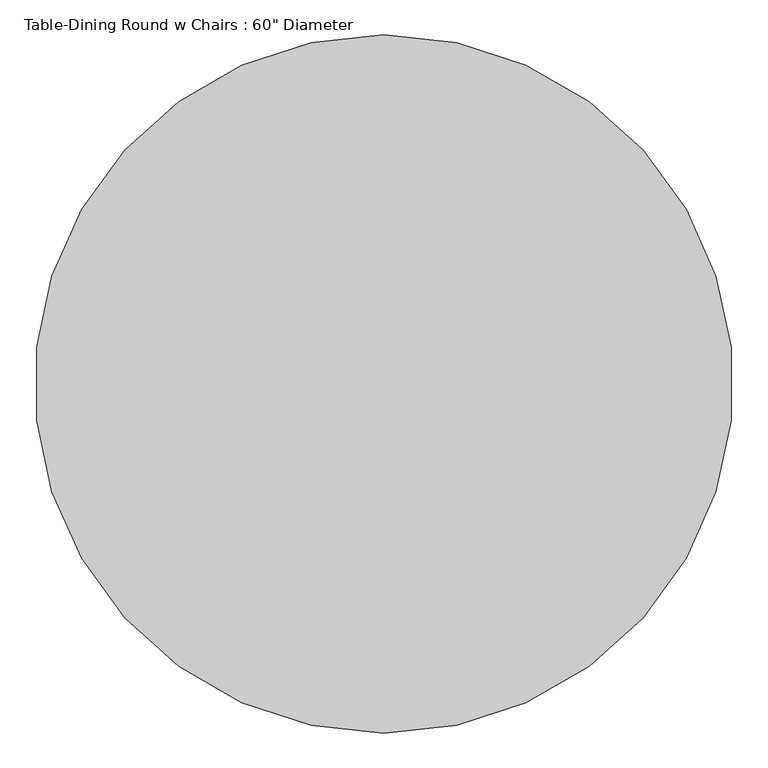
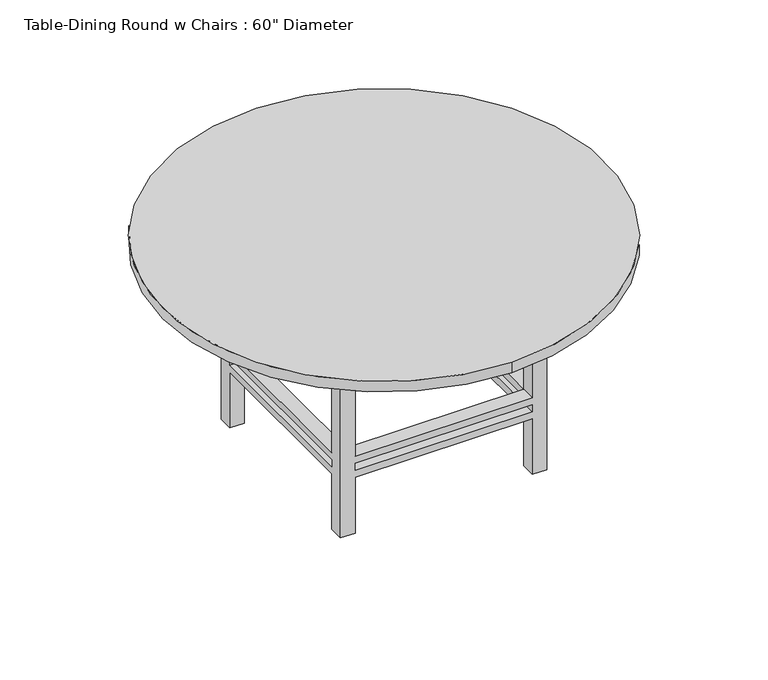
"""IFC4 building model written with IfcOpenShell, lengths in millimetres: furniture geometry."""

from ifc_helpers import new_model, si_unit, point, frame, frame_2d, origin, place, context, project, spatial, polyline, circle_curve, trimmed, segment, composite_curve, outline, extrude, faceted_brep, source, transform, mapped, element, save


def furniture_86cdcdde(model_context):
    return source(origin(), model_context, "Body", "SolidModel", [
        extrude(outline(polyline([(484.6819672, 196.1213115), (484.6819672, -565.8786885), (-277.3180328, -565.8786885), (-277.3180328, 196.1213115), (484.6819672, 196.1213115)]), holes=[polyline([(459.2819672, 170.7213115), (-251.9180328, 170.7213115), (-251.9180328, -540.4786885), (459.2819672, -540.4786885), (459.2819672, 170.7213115)])]), frame((0.0, 0.0, 647.7), z_axis=(0.0, 0.0, 1.0), x_axis=(1.0, 0.0, 0.0)), (0.0, 0.0, 1.0), 76.2),
        faceted_brep([(408.4819672, 119.9213115, 279.4), (408.4819672, -489.6786885, 279.4), (459.2819672, -489.6786885, 279.4), (459.2819672, 119.9213115, 279.4), (-201.1180328, -489.6786885, 279.4), (-201.1180328, -540.4786885, 279.4), (408.4819672, -540.4786885, 279.4), (-201.1180328, 119.9213115, 279.4), (-251.9180328, 119.9213115, 279.4), (-251.9180328, -489.6786885, 279.4), (408.4819672, 170.7213115, 279.4), (-201.1180328, 170.7213115, 279.4), (408.4819672, 119.9213115, 254.0), (-201.1180328, 119.9213115, 254.0), (-201.1180328, 170.7213115, 254.0), (408.4819672, 170.7213115, 254.0), (-201.1180328, -489.6786885, 254.0), (-251.9180328, -489.6786885, 254.0), (-251.9180328, 119.9213115, 254.0), (408.4819672, -489.6786885, 254.0), (408.4819672, -540.4786885, 254.0), (-201.1180328, -540.4786885, 254.0), (459.2819672, 119.9213115, 254.0), (459.2819672, -489.6786885, 254.0), (-251.9180328, 170.7213115, 647.7), (-201.1180328, 170.7213115, 647.7), (408.4819672, 170.7213115, 647.7), (459.2819672, 170.7213115, 647.7), (459.2819672, 170.7213115, 0.0), (408.4819672, 170.7213115, 0.0), (408.4819672, 170.7213115, 203.2), (-201.1180328, 170.7213115, 203.2), (-201.1180328, 170.7213115, 0.0), (-251.9180328, 170.7213115, 0.0), (-201.1180328, 170.7213115, 228.6), (408.4819672, 170.7213115, 228.6), (-251.9180328, 119.9213115, 647.7), (-251.9180328, 119.9213115, 0.0), (-251.9180328, 119.9213115, 203.2), (-251.9180328, -489.6786885, 203.2), (-251.9180328, -489.6786885, 0.0), (-251.9180328, -540.4786885, 0.0), (-251.9180328, -540.4786885, 647.7), (-251.9180328, -489.6786885, 647.7), (-251.9180328, -489.6786885, 228.6), (-251.9180328, 119.9213115, 228.6), (459.2819672, -540.4786885, 647.7), (408.4819672, -540.4786885, 647.7), (-201.1180328, -540.4786885, 647.7), (-201.1180328, -540.4786885, 0.0), (-201.1180328, -540.4786885, 203.2), (408.4819672, -540.4786885, 203.2), (408.4819672, -540.4786885, 0.0), (459.2819672, -540.4786885, 0.0), (408.4819672, -540.4786885, 228.6), (-201.1180328, -540.4786885, 228.6), (459.2819672, 119.9213115, 647.7), (459.2819672, -489.6786885, 647.7), (459.2819672, -489.6786885, 0.0), (459.2819672, -489.6786885, 203.2), (459.2819672, 119.9213115, 203.2), (459.2819672, 119.9213115, 0.0), (459.2819672, 119.9213115, 228.6), (459.2819672, -489.6786885, 228.6), (-201.1180328, 119.9213115, 647.7), (408.4819672, -489.6786885, 647.7), (408.4819672, 119.9213115, 647.7), (-201.1180328, -489.6786885, 647.7), (408.4819672, 119.9213115, 0.0), (-201.1180328, -489.6786885, 0.0), (-201.1180328, 119.9213115, 0.0), (408.4819672, -489.6786885, 0.0), (-201.1180328, 119.9213115, 228.6), (-201.1180328, 119.9213115, 203.2), (408.4819672, 119.9213115, 228.6), (408.4819672, 119.9213115, 203.2), (408.4819672, -489.6786885, 228.6), (408.4819672, -489.6786885, 203.2), (-201.1180328, -489.6786885, 228.6), (-201.1180328, -489.6786885, 203.2)], [[[0, 1, 2, 3]], [[1, 4, 5, 6]], [[4, 7, 8, 9]], [[7, 0, 10, 11]], [[12, 13, 14, 15]], [[13, 16, 17, 18]], [[16, 19, 20, 21]], [[19, 12, 22, 23]], [[24, 25, 11, 10, 26, 27, 28, 29, 30, 31, 32, 33], [14, 34, 35, 15]], [[36, 24, 33, 37, 38, 39, 40, 41, 42, 43, 9, 8], [17, 44, 45, 18]], [[46, 47, 6, 5, 48, 42, 41, 49, 50, 51, 52, 53], [20, 54, 55, 21]], [[28, 27, 56, 3, 2, 57, 46, 53, 58, 59, 60, 61], [22, 62, 63, 23]], [[1, 0, 12, 19]], [[4, 1, 19, 16]], [[7, 4, 16, 13]], [[0, 7, 13, 12]], [[25, 24, 36, 64]], [[47, 46, 57, 65]], [[26, 66, 56, 27]], [[48, 67, 43, 42]], [[29, 28, 61, 68]], [[49, 41, 40, 69]], [[32, 70, 37, 33]], [[52, 71, 58, 53]], [[13, 18, 45, 72]], [[64, 36, 8, 7]], [[37, 70, 73, 38]], [[14, 13, 72, 34]], [[25, 64, 7, 11]], [[70, 32, 31, 73]], [[12, 15, 35, 74]], [[66, 26, 10, 0]], [[29, 68, 75, 30]], [[22, 12, 74, 62]], [[56, 66, 0, 3]], [[68, 61, 60, 75]], [[19, 23, 63, 76]], [[65, 57, 2, 1]], [[58, 71, 77, 59]], [[20, 19, 76, 54]], [[47, 65, 1, 6]], [[71, 52, 51, 77]], [[16, 21, 55, 78]], [[67, 48, 5, 4]], [[49, 69, 79, 50]], [[17, 16, 78, 44]], [[43, 67, 4, 9]], [[69, 40, 39, 79]], [[74, 76, 63, 62]], [[76, 78, 55, 54]], [[78, 72, 45, 44]], [[72, 74, 35, 34]], [[75, 73, 31, 30]], [[73, 79, 39, 38]], [[79, 77, 51, 50]], [[77, 75, 60, 59]], [[76, 74, 75, 77]], [[78, 76, 77, 79]], [[72, 78, 79, 73]], [[74, 72, 73, 75]]]),
        extrude(outline(composite_curve([segment(trimmed(circle_curve(frame_2d((103.6819672, -184.8786885)), 762.0), [point((103.6819672, -946.8786885))], [point((103.6819672, 577.1213115))], False, "CARTESIAN"), True, "CONTINUOUS"), segment(trimmed(circle_curve(frame_2d((103.6819672, -184.8786885)), 762.0), [point((103.6819672, 577.1213115))], [point((103.6819672, -946.8786885))], False, "CARTESIAN"), True, "CONTINUOUS")], self_intersect=False)), frame((0.0, 0.0, 723.9), z_axis=(0.0, 0.0, 1.0), x_axis=(1.0, 0.0, 0.0)), (0.0, 0.0, 1.0), 38.1),
    ])


if __name__ == "__main__":
    model = new_model("IFC4")
    model_context = context("Model", 3, world=origin())
    ifc_project = project(units=[si_unit("LENGTHUNIT", "METRE", prefix="MILLI")], contexts=[model_context])
    site = spatial("IfcSite", under=ifc_project)
    building = spatial("IfcBuilding", under=site)
    placement = place(None, origin())
    furniture_shape = furniture_86cdcdde(model_context)
    element("IfcFurniture", 1, ObjectType="Table-Dining Round w Chairs : 60\" Diameter", at=placement, inside=building, context=model_context, shape_type="MappedRepresentation", body=[
        mapped(furniture_shape, transform((0.0, 0.0, 0.0), x_axis=(1.0, 0.0, 0.0), y_axis=(0.0, 1.0, 0.0), z_axis=(0.0, 0.0, 1.0))),
    ])
    save(model, "model.ifc")

# Revit data of these elements
# Type "Table-Dining Round w Chairs : 60\" Diameter"
#   Assembly Code = "E2020200"
#   Radius = 2' - 6"
#   Diameter = 5' - 0"
#   Height = 2' - 6"
#   Chairs = 6
#   Base Material = Pine
#   Top Material = Laminate, Linen, Matte
#   Default Elevation = 0
# Element 1 (IfcFurniture, "Table-Dining Round w Chairs : 60\" Diameter")
#   Materials on its faces: "Pine", "Laminate, Linen, Matte"
# Materials
#   "Pine": class "Wood", colour RGB 223 192 134, transparency 0, Description = "Pinus Echinata", Cost = 0
#   "Laminate, Linen, Matte": class "Plastic", colour RGB 198 189 176, transparency 0, Description = "Plastic Laminate - Linen, Matte", Cost = 0
